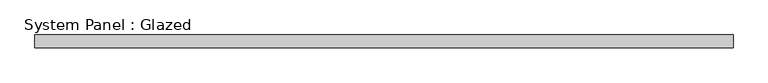
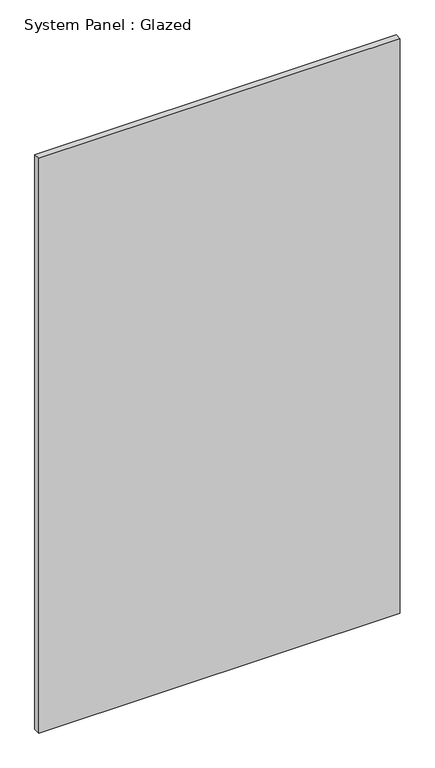
"""IFC4 building model written with IfcOpenShell, lengths in millimetres: plate geometry, System Panel : Glazed."""

from ifc_helpers import new_model, si_unit, origin, origin_with_axes, place, context, project, spatial, polyline, outline, extrude, source, transform, mapped, element, save


def system_panel_glazed_1fb160e7(model_context):
    return source(origin(), model_context, "Body", "SweptSolid", [
        extrude(outline(polyline([(697.4416667, 19.05), (-697.4416667, 19.05), (-697.4416667, 44.45), (697.4416667, 44.45), (697.4416667, 19.05)])), origin_with_axes(), (0.0, 0.0, 1.0), 2343.15),
    ])


if __name__ == "__main__":
    model = new_model("IFC4")
    model_context = context("Model", 3, world=origin())
    ifc_project = project(units=[si_unit("LENGTHUNIT", "METRE", prefix="MILLI")], contexts=[model_context])
    site = spatial("IfcSite", under=ifc_project)
    building = spatial("IfcBuilding", under=site)
    placement = place(None, origin())
    system_panel_glazed_shape = system_panel_glazed_1fb160e7(model_context)
    element("IfcPlate", 1, ObjectType="System Panel : Glazed", at=placement, inside=building, context=model_context, shape_type="MappedRepresentation", body=[
        mapped(system_panel_glazed_shape, transform((0.0, 0.0, 0.0), x_axis=(1.0, 0.0, 0.0), y_axis=(0.0, 1.0, 0.0), z_axis=(0.0, 0.0, 1.0))),
    ])
    save(model, "model.ifc")

# Revit data of these elements
# Type "System Panel : Glazed"
#   Construction Type Id = "GSP4R"
#   Analytic Construction = "1/8 in Pilkington single glazing"
#   Visual Light Transmittance = 0.9
#   Solar Heat Gain Coefficient = 0.86
#   Heat Transfer Coefficient (U) = 1.18115 BTU/(h·ft²·°F)
# Element 1 (IfcPlate, "System Panel : Glazed")
#   Materials on its faces: "Glass"
# Materials
#   "Glass": class "Glass", colour RGB 0 128 192, transparency 0.75, Description = "Soda Lime Glass", Cost = 0
